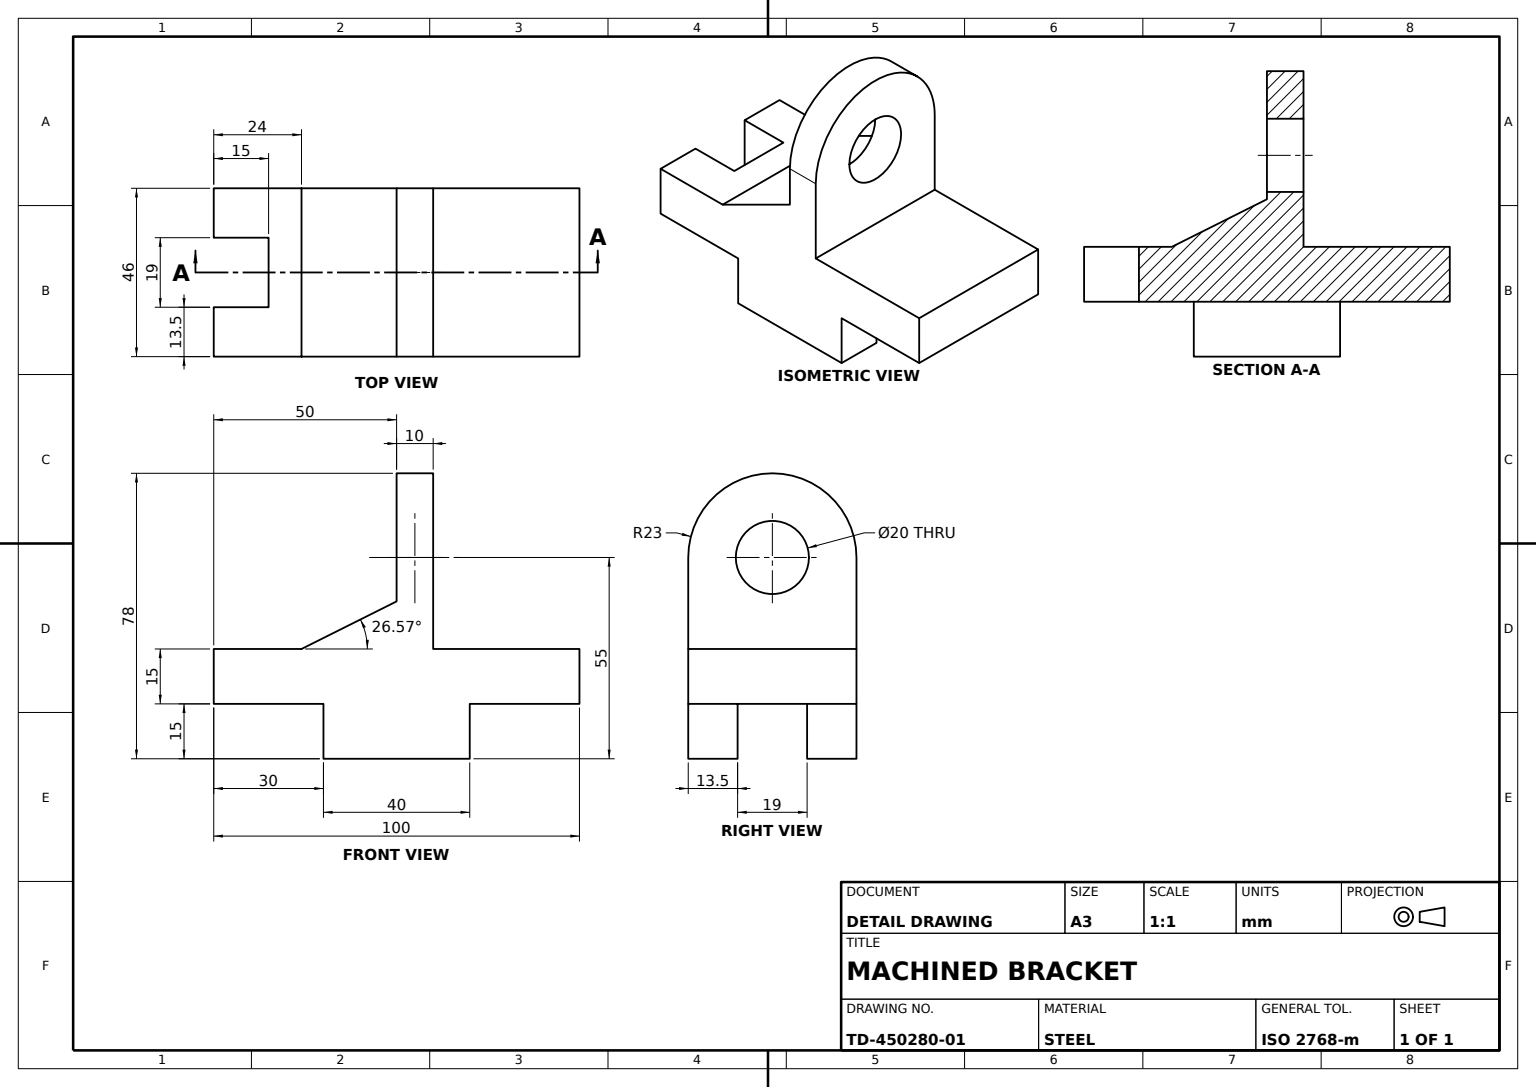
SolidWorks part; units mm, degrees
material "Plain Carbon Steel"
ref_plane "Front Plane" through (0, 0, 0) normal (0, 0, 1) x (1, 0, 0)
ref_plane "Top Plane" through (0, 0, 0) normal (0, 1, 0) x (1, 0, 0)
ref_plane "Right Plane" through (0, 0, 0) normal (1, 0, 0) x (0, 0, -1)
sketch "Base Profile Sketch" plane through (0, 0, 0) normal (1, 0, 0) x (0, 0, -1)
  line L0 (-60, 0) -> (40, 0)
  line L1 (-60, 0) -> (-60, -15)
  line L2 (-60, -15) -> (-30, -15)
  line L3 (-30, -15) -> (-30, -30)
  line L4 (-30, -30) -> (10, -30)
  line L5 (10, -30) -> (10, -15)
  line L6 (10, -15) -> (40, -15)
  line L7 (40, -15) -> (40, 0)
  dimension "D1" = 100
  dimension "D2" = 30
  dimension "D3" = 15
  dimension "D4" = 30
  dimension "D5" = 40
  dimension "D6" = 40
extrude "Base Body" add sketch "Base Profile Sketch" along normal mid plane 46
sketch "Fork Slot Sketch" plane through (0, 0, 0) normal (0, 1, 0) x (1, 0, 0)
  line L0 (23, -60) -> (-23, -60) construction
  line L1 (-9.5, -60) -> (9.5, -60)
  line L2 (-9.5, -60) -> (-9.5, -45)
  line L3 (-9.5, -45) -> (9.5, -45)
  line L4 (9.5, -60) -> (9.5, -45)
  point P6 (0, -60)
  dimension "D1" = 19
  dimension "D2" = 15
extrude "Fork Slot 19x15" cut sketch "Fork Slot Sketch" against normal up to next
sketch "Channel Cut Sketch" plane through (0, -30, 0) normal (0, -1, 0) x (1, 0, 0)
  line L0 (0, 30) -> (0, -10)
  line L1 (23, 30) -> (-23, 30) construction
  line L2 (23, -10) -> (-23, -10) construction
extrude "Thin Channel Cut 19" cut sketch "Channel Cut Sketch" against normal up to surface (15 mm away) thin up to face at (0, -15, -25) thin type mid plane wall 19
sketch "Lug Sketch" plane through (0, 0, 0) normal (0, 0, 1) x (1, 0, 0)
  line L0 (-9.5, -30) -> (-23, -30) construction
  line L1 (23, 25) -> (23, 0)
  line L2 (23, 0) -> (9.5, 0) construction
  line L3 (-23, 25) -> (-23, 0)
  line L4 (-9.5, 0) -> (-23, 0) construction
  line L5 (-23, 0) -> (23, 0)
  circle A0 centre (0, 25) radius 10
  arc A1 (23, 25) -> (-23, 25) centre (0, 25) ccw
  dimension "D2" = 23
  dimension "D3" = 20
  dimension "D1" = 55
extrude "Lug with Bore" add sketch "Lug Sketch" along normal blind 10 contours A1 L3 L5 L1 | A0
sketch "Support Rib Sketch" plane through (0, 0, 0) normal (1, 0, 0) x (0, 0, -1)
  line L0 (-10, 13) -> (-36, 0)
  line L1 (-10, 25) -> (-10, 0) construction
  line L2 (-10, 0) -> (-60, 0) construction
  line L3 (-60, 0) -> (-60, -15) construction
  dimension "D1" = 13
  dimension "D2" = 24
rib "Support Rib" sketch "Support Rib Sketch" sketch "Support Rib Sketch" thickness 46 extrusion direction parallel to sketch draft on no parameters "D1"=46
